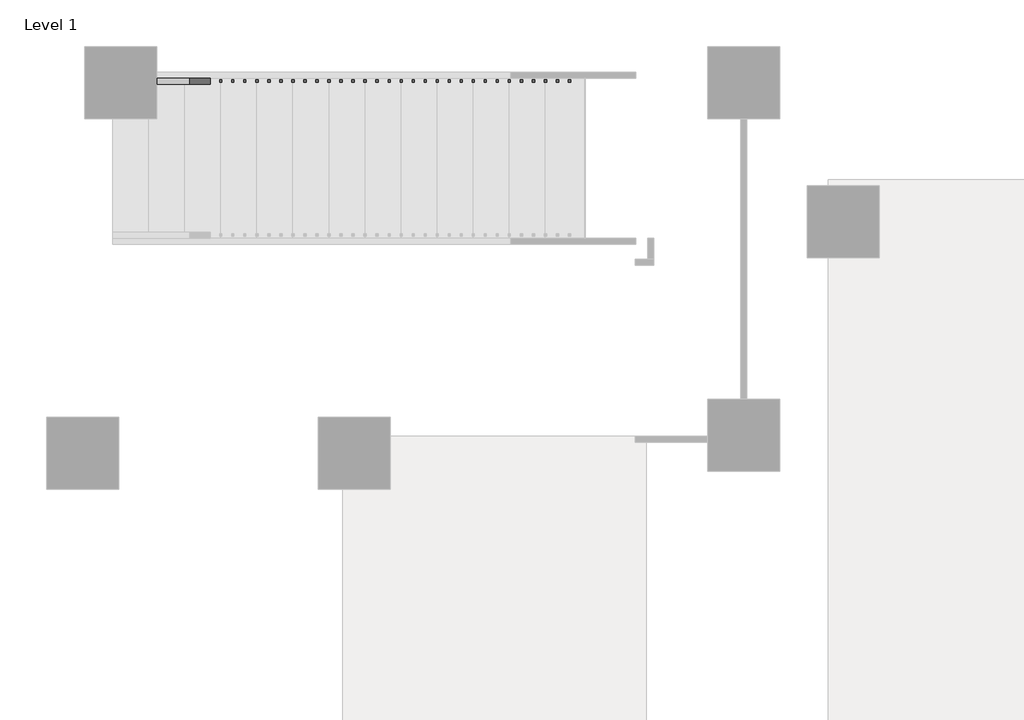
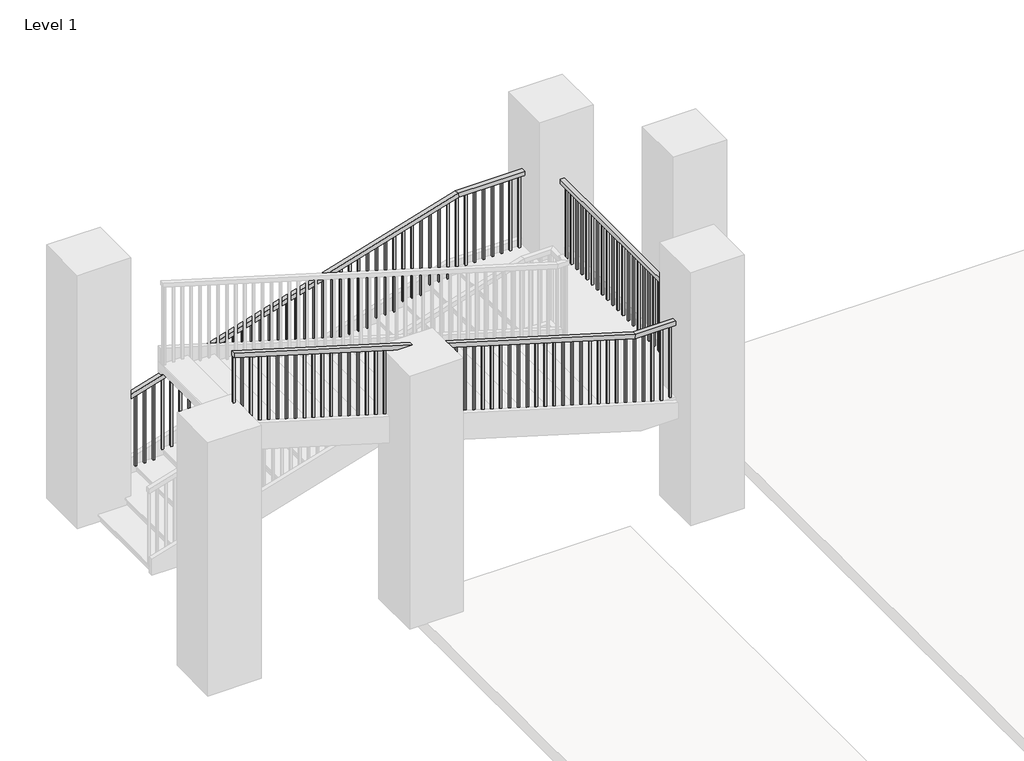
# One storey, part 5 of 6: 1 railing.
"""IFC4 building model written with IfcOpenShell, lengths in millimetres."""

from ifc_helpers import new_model, si_unit, frame, origin, place, context, project, spatial, polyline, outline, extrude, faceted_brep, element, save

model = new_model("IFC4")

# Units and contexts
model_context = context("Model", 3, world=origin())
ifc_project = project(units=[si_unit("LENGTHUNIT", "METRE", prefix="MILLI")], contexts=[model_context])

# Site, building, storey
site = spatial("IfcSite", under=ifc_project)
building = spatial("IfcBuilding", under=site)
storey = spatial("IfcBuildingStorey", under=building, Name="Level 1", Elevation=0.0)

# Railing
placement = place(None, origin())
element("IfcRailing", 1, ObjectType="Handrail - Rectangular", at=placement, inside=storey, context=model_context, shape_type="SolidModel", body=[
    faceted_brep([(-5254.0891351, 12506.0715905, 1005.84), (-5254.0891351, 12506.0715905, 952.8032429), (-5254.0891351, 12455.2715905, 952.8032429), (-5254.0891351, 12455.2715905, 1005.84), (-986.8891351, 12506.0715905, 2286.0), (-979.4332782, 12506.0715905, 2235.2), (-979.4332782, 12455.2715905, 2235.2), (-986.8891351, 12455.2715905, 2286.0), (54.5108649, 12506.0715905, 2286.0), (54.5108649, 12506.0715905, 2235.2), (3.7108649, 12455.2715905, 2235.2), (3.7108649, 12455.2715905, 2286.0), (54.5108649, 9478.4949943, 2286.0), (54.5108649, 9478.4949943, 2235.2), (3.7108649, 9529.2949943, 2235.2), (3.7108649, 9529.2949943, 2286.0), (-682.0891351, 9478.4949943, 2286.0), (-689.544992, 9478.4949943, 2235.2), (-689.544992, 9529.2949943, 2235.2), (-682.0891351, 9529.2949943, 2286.0), (-5254.0891351, 9478.4949943, 3657.6), (-5254.0891351, 9529.2949943, 3657.6), (-5254.0891351, 9529.2949943, 3604.5632429), (-5254.0891351, 9478.4949943, 3604.5632429)], [[[0, 1, 2, 3]], [[1, 0, 4, 5]], [[2, 1, 5, 6]], [[3, 2, 6, 7]], [[0, 3, 7, 4]], [[5, 4, 8, 9]], [[6, 5, 9, 10]], [[7, 6, 10, 11]], [[4, 7, 11, 8]], [[9, 8, 12, 13]], [[10, 9, 13, 14]], [[11, 10, 14, 15]], [[8, 11, 15, 12]], [[13, 12, 16, 17]], [[14, 13, 17, 18]], [[15, 14, 18, 19]], [[12, 15, 19, 16]], [[20, 21, 22, 23]], [[17, 16, 20, 23]], [[18, 17, 23, 22]], [[19, 18, 22, 21]], [[16, 19, 21, 20]]]),
    extrude(outline(polyline([(3576.9407429, -5162.0141351), (2651.76, -5162.0141351), (2651.76, -5142.9641351), (3571.2257429, -5142.9641351), (3576.9407429, -5162.0141351)])), frame((0.0, 9494.3699943, 0.0), z_axis=(0.0, 1.0, 0.0), x_axis=(0.0, 0.0, 1.0)), (0.0, 0.0, 1.0), 19.05),
    extrude(outline(polyline([(3546.4607429, -5060.4141351), (2651.76, -5060.4141351), (2651.76, -5041.3641351), (3540.7457429, -5041.3641351), (3546.4607429, -5060.4141351)])), frame((0.0, 9494.3699943, 0.0), z_axis=(0.0, 1.0, 0.0), x_axis=(0.0, 0.0, 1.0)), (0.0, 0.0, 1.0), 19.05),
    extrude(outline(polyline([(3515.9807429, -4958.8141351), (2651.76, -4958.8141351), (2651.76, -4939.7641351), (3510.2657429, -4939.7641351), (3515.9807429, -4958.8141351)])), frame((0.0, 9494.3699943, 0.0), z_axis=(0.0, 1.0, 0.0), x_axis=(0.0, 0.0, 1.0)), (0.0, 0.0, 1.0), 19.05),
    extrude(outline(polyline([(3485.5007429, -4857.2141351), (2560.32, -4857.2141351), (2560.32, -4838.1641351), (3479.7857429, -4838.1641351), (3485.5007429, -4857.2141351)])), frame((0.0, 9494.3699943, 0.0), z_axis=(0.0, 1.0, 0.0), x_axis=(0.0, 0.0, 1.0)), (0.0, 0.0, 1.0), 19.05),
    extrude(outline(polyline([(3455.0207429, -4755.6141351), (2560.32, -4755.6141351), (2560.32, -4736.5641351), (3449.3057429, -4736.5641351), (3455.0207429, -4755.6141351)])), frame((0.0, 9494.3699943, 0.0), z_axis=(0.0, 1.0, 0.0), x_axis=(0.0, 0.0, 1.0)), (0.0, 0.0, 1.0), 19.05),
    extrude(outline(polyline([(3424.5407429, -4654.0141351), (2560.32, -4654.0141351), (2560.32, -4634.9641351), (3418.8257429, -4634.9641351), (3424.5407429, -4654.0141351)])), frame((0.0, 9494.3699943, 0.0), z_axis=(0.0, 1.0, 0.0), x_axis=(0.0, 0.0, 1.0)), (0.0, 0.0, 1.0), 19.05),
    extrude(outline(polyline([(3394.0607429, -4552.4141351), (2468.88, -4552.4141351), (2468.88, -4533.3641351), (3388.3457429, -4533.3641351), (3394.0607429, -4552.4141351)])), frame((0.0, 9494.3699943, 0.0), z_axis=(0.0, 1.0, 0.0), x_axis=(0.0, 0.0, 1.0)), (0.0, 0.0, 1.0), 19.05),
    extrude(outline(polyline([(3363.5807429, -4450.8141351), (2468.88, -4450.8141351), (2468.88, -4431.7641351), (3357.8657429, -4431.7641351), (3363.5807429, -4450.8141351)])), frame((0.0, 9494.3699943, 0.0), z_axis=(0.0, 1.0, 0.0), x_axis=(0.0, 0.0, 1.0)), (0.0, 0.0, 1.0), 19.05),
    extrude(outline(polyline([(3333.1007429, -4349.2141351), (2468.88, -4349.2141351), (2468.88, -4330.1641351), (3327.3857429, -4330.1641351), (3333.1007429, -4349.2141351)])), frame((0.0, 9494.3699943, 0.0), z_axis=(0.0, 1.0, 0.0), x_axis=(0.0, 0.0, 1.0)), (0.0, 0.0, 1.0), 19.05),
    extrude(outline(polyline([(3302.6207429, -4247.6141351), (2377.44, -4247.6141351), (2377.44, -4228.5641351), (3296.9057429, -4228.5641351), (3302.6207429, -4247.6141351)])), frame((0.0, 9494.3699943, 0.0), z_axis=(0.0, 1.0, 0.0), x_axis=(0.0, 0.0, 1.0)), (0.0, 0.0, 1.0), 19.05),
    extrude(outline(polyline([(3272.1407429, -4146.0141351), (2377.44, -4146.0141351), (2377.44, -4126.9641351), (3266.4257429, -4126.9641351), (3272.1407429, -4146.0141351)])), frame((0.0, 9494.3699943, 0.0), z_axis=(0.0, 1.0, 0.0), x_axis=(0.0, 0.0, 1.0)), (0.0, 0.0, 1.0), 19.05),
    extrude(outline(polyline([(3241.6607429, -4044.4141351), (2377.44, -4044.4141351), (2377.44, -4025.3641351), (3235.9457429, -4025.3641351), (3241.6607429, -4044.4141351)])), frame((0.0, 9494.3699943, 0.0), z_axis=(0.0, 1.0, 0.0), x_axis=(0.0, 0.0, 1.0)), (0.0, 0.0, 1.0), 19.05),
    extrude(outline(polyline([(3211.1807429, -3942.8141351), (2286.0, -3942.8141351), (2286.0, -3923.7641351), (3205.4657429, -3923.7641351), (3211.1807429, -3942.8141351)])), frame((0.0, 9494.3699943, 0.0), z_axis=(0.0, 1.0, 0.0), x_axis=(0.0, 0.0, 1.0)), (0.0, 0.0, 1.0), 19.05),
    extrude(outline(polyline([(3180.7007429, -3841.2141351), (2286.0, -3841.2141351), (2286.0, -3822.1641351), (3174.9857429, -3822.1641351), (3180.7007429, -3841.2141351)])), frame((0.0, 9494.3699943, 0.0), z_axis=(0.0, 1.0, 0.0), x_axis=(0.0, 0.0, 1.0)), (0.0, 0.0, 1.0), 19.05),
    extrude(outline(polyline([(3150.2207429, -3739.6141351), (2286.0, -3739.6141351), (2286.0, -3720.5641351), (3144.5057429, -3720.5641351), (3150.2207429, -3739.6141351)])), frame((0.0, 9494.3699943, 0.0), z_axis=(0.0, 1.0, 0.0), x_axis=(0.0, 0.0, 1.0)), (0.0, 0.0, 1.0), 19.05),
    extrude(outline(polyline([(3119.7407429, -3638.0141351), (2194.56, -3638.0141351), (2194.56, -3618.9641351), (3114.0257429, -3618.9641351), (3119.7407429, -3638.0141351)])), frame((0.0, 9494.3699943, 0.0), z_axis=(0.0, 1.0, 0.0), x_axis=(0.0, 0.0, 1.0)), (0.0, 0.0, 1.0), 19.05),
    extrude(outline(polyline([(3089.2607429, -3536.4141351), (2194.56, -3536.4141351), (2194.56, -3517.3641351), (3083.5457429, -3517.3641351), (3089.2607429, -3536.4141351)])), frame((0.0, 9494.3699943, 0.0), z_axis=(0.0, 1.0, 0.0), x_axis=(0.0, 0.0, 1.0)), (0.0, 0.0, 1.0), 19.05),
    extrude(outline(polyline([(3058.7807429, -3434.8141351), (2194.56, -3434.8141351), (2194.56, -3415.7641351), (3053.0657429, -3415.7641351), (3058.7807429, -3434.8141351)])), frame((0.0, 9494.3699943, 0.0), z_axis=(0.0, 1.0, 0.0), x_axis=(0.0, 0.0, 1.0)), (0.0, 0.0, 1.0), 19.05),
    extrude(outline(polyline([(3028.3007429, -3333.2141351), (2103.12, -3333.2141351), (2103.12, -3314.1641351), (3022.5857429, -3314.1641351), (3028.3007429, -3333.2141351)])), frame((0.0, 9494.3699943, 0.0), z_axis=(0.0, 1.0, 0.0), x_axis=(0.0, 0.0, 1.0)), (0.0, 0.0, 1.0), 19.05),
    extrude(outline(polyline([(2997.8207429, -3231.6141351), (2103.12, -3231.6141351), (2103.12, -3212.5641351), (2992.1057429, -3212.5641351), (2997.8207429, -3231.6141351)])), frame((0.0, 9494.3699943, 0.0), z_axis=(0.0, 1.0, 0.0), x_axis=(0.0, 0.0, 1.0)), (0.0, 0.0, 1.0), 19.05),
    extrude(outline(polyline([(2967.3407429, -3130.0141351), (2103.12, -3130.0141351), (2103.12, -3110.9641351), (2961.6257429, -3110.9641351), (2967.3407429, -3130.0141351)])), frame((0.0, 9494.3699943, 0.0), z_axis=(0.0, 1.0, 0.0), x_axis=(0.0, 0.0, 1.0)), (0.0, 0.0, 1.0), 19.05),
    extrude(outline(polyline([(2936.8607429, -3028.4141351), (2011.68, -3028.4141351), (2011.68, -3009.3641351), (2931.1457429, -3009.3641351), (2936.8607429, -3028.4141351)])), frame((0.0, 9494.3699943, 0.0), z_axis=(0.0, 1.0, 0.0), x_axis=(0.0, 0.0, 1.0)), (0.0, 0.0, 1.0), 19.05),
    extrude(outline(polyline([(2906.3807429, -2926.8141351), (2011.68, -2926.8141351), (2011.68, -2907.7641351), (2900.6657429, -2907.7641351), (2906.3807429, -2926.8141351)])), frame((0.0, 9494.3699943, 0.0), z_axis=(0.0, 1.0, 0.0), x_axis=(0.0, 0.0, 1.0)), (0.0, 0.0, 1.0), 19.05),
    extrude(outline(polyline([(2875.9007429, -2825.2141351), (2011.68, -2825.2141351), (2011.68, -2806.1641351), (2870.1857429, -2806.1641351), (2875.9007429, -2825.2141351)])), frame((0.0, 9494.3699943, 0.0), z_axis=(0.0, 1.0, 0.0), x_axis=(0.0, 0.0, 1.0)), (0.0, 0.0, 1.0), 19.05),
    extrude(outline(polyline([(2845.4207429, -2723.6141351), (1920.24, -2723.6141351), (1920.24, -2704.5641351), (2839.7057429, -2704.5641351), (2845.4207429, -2723.6141351)])), frame((0.0, 9494.3699943, 0.0), z_axis=(0.0, 1.0, 0.0), x_axis=(0.0, 0.0, 1.0)), (0.0, 0.0, 1.0), 19.05),
    extrude(outline(polyline([(2814.9407429, -2622.0141351), (1920.24, -2622.0141351), (1920.24, -2602.9641351), (2809.2257429, -2602.9641351), (2814.9407429, -2622.0141351)])), frame((0.0, 9494.3699943, 0.0), z_axis=(0.0, 1.0, 0.0), x_axis=(0.0, 0.0, 1.0)), (0.0, 0.0, 1.0), 19.05),
    extrude(outline(polyline([(2784.4607429, -2520.4141351), (1920.24, -2520.4141351), (1920.24, -2501.3641351), (2778.7457429, -2501.3641351), (2784.4607429, -2520.4141351)])), frame((0.0, 9494.3699943, 0.0), z_axis=(0.0, 1.0, 0.0), x_axis=(0.0, 0.0, 1.0)), (0.0, 0.0, 1.0), 19.05),
    extrude(outline(polyline([(2753.9807429, -2418.8141351), (1828.8, -2418.8141351), (1828.8, -2399.7641351), (2748.2657429, -2399.7641351), (2753.9807429, -2418.8141351)])), frame((0.0, 9494.3699943, 0.0), z_axis=(0.0, 1.0, 0.0), x_axis=(0.0, 0.0, 1.0)), (0.0, 0.0, 1.0), 19.05),
    extrude(outline(polyline([(2723.5007429, -2317.2141351), (1828.8, -2317.2141351), (1828.8, -2298.1641351), (2717.7857429, -2298.1641351), (2723.5007429, -2317.2141351)])), frame((0.0, 9494.3699943, 0.0), z_axis=(0.0, 1.0, 0.0), x_axis=(0.0, 0.0, 1.0)), (0.0, 0.0, 1.0), 19.05),
    extrude(outline(polyline([(2693.0207429, -2215.6141351), (1828.8, -2215.6141351), (1828.8, -2196.5641351), (2687.3057429, -2196.5641351), (2693.0207429, -2215.6141351)])), frame((0.0, 9494.3699943, 0.0), z_axis=(0.0, 1.0, 0.0), x_axis=(0.0, 0.0, 1.0)), (0.0, 0.0, 1.0), 19.05),
    extrude(outline(polyline([(2662.5407429, -2114.0141351), (1737.36, -2114.0141351), (1737.36, -2094.9641351), (2656.8257429, -2094.9641351), (2662.5407429, -2114.0141351)])), frame((0.0, 9494.3699943, 0.0), z_axis=(0.0, 1.0, 0.0), x_axis=(0.0, 0.0, 1.0)), (0.0, 0.0, 1.0), 19.05),
    extrude(outline(polyline([(2632.0607429, -2012.4141351), (1737.36, -2012.4141351), (1737.36, -1993.3641351), (2626.3457429, -1993.3641351), (2632.0607429, -2012.4141351)])), frame((0.0, 9494.3699943, 0.0), z_axis=(0.0, 1.0, 0.0), x_axis=(0.0, 0.0, 1.0)), (0.0, 0.0, 1.0), 19.05),
    extrude(outline(polyline([(2601.5807429, -1910.8141351), (1737.36, -1910.8141351), (1737.36, -1891.7641351), (2595.8657429, -1891.7641351), (2601.5807429, -1910.8141351)])), frame((0.0, 9494.3699943, 0.0), z_axis=(0.0, 1.0, 0.0), x_axis=(0.0, 0.0, 1.0)), (0.0, 0.0, 1.0), 19.05),
    extrude(outline(polyline([(2571.1007429, -1809.2141351), (1645.92, -1809.2141351), (1645.92, -1790.1641351), (2565.3857429, -1790.1641351), (2571.1007429, -1809.2141351)])), frame((0.0, 9494.3699943, 0.0), z_axis=(0.0, 1.0, 0.0), x_axis=(0.0, 0.0, 1.0)), (0.0, 0.0, 1.0), 19.05),
    extrude(outline(polyline([(2540.6207429, -1707.6141351), (1645.92, -1707.6141351), (1645.92, -1688.5641351), (2534.9057429, -1688.5641351), (2540.6207429, -1707.6141351)])), frame((0.0, 9494.3699943, 0.0), z_axis=(0.0, 1.0, 0.0), x_axis=(0.0, 0.0, 1.0)), (0.0, 0.0, 1.0), 19.05),
    extrude(outline(polyline([(2510.1407429, -1606.0141351), (1645.92, -1606.0141351), (1645.92, -1586.9641351), (2504.4257429, -1586.9641351), (2510.1407429, -1606.0141351)])), frame((0.0, 9494.3699943, 0.0), z_axis=(0.0, 1.0, 0.0), x_axis=(0.0, 0.0, 1.0)), (0.0, 0.0, 1.0), 19.05),
    extrude(outline(polyline([(2479.6607429, -1504.4141351), (1554.48, -1504.4141351), (1554.48, -1485.3641351), (2473.9457429, -1485.3641351), (2479.6607429, -1504.4141351)])), frame((0.0, 9494.3699943, 0.0), z_axis=(0.0, 1.0, 0.0), x_axis=(0.0, 0.0, 1.0)), (0.0, 0.0, 1.0), 19.05),
    extrude(outline(polyline([(2449.1807429, -1402.8141351), (1554.48, -1402.8141351), (1554.48, -1383.7641351), (2443.4657429, -1383.7641351), (2449.1807429, -1402.8141351)])), frame((0.0, 9494.3699943, 0.0), z_axis=(0.0, 1.0, 0.0), x_axis=(0.0, 0.0, 1.0)), (0.0, 0.0, 1.0), 19.05),
    extrude(outline(polyline([(2418.7007429, -1301.2141351), (1554.48, -1301.2141351), (1554.48, -1282.1641351), (2412.9857429, -1282.1641351), (2418.7007429, -1301.2141351)])), frame((0.0, 9494.3699943, 0.0), z_axis=(0.0, 1.0, 0.0), x_axis=(0.0, 0.0, 1.0)), (0.0, 0.0, 1.0), 19.05),
    extrude(outline(polyline([(2388.2207429, -1199.6141351), (1463.04, -1199.6141351), (1463.04, -1180.5641351), (2382.5057429, -1180.5641351), (2388.2207429, -1199.6141351)])), frame((0.0, 9494.3699943, 0.0), z_axis=(0.0, 1.0, 0.0), x_axis=(0.0, 0.0, 1.0)), (0.0, 0.0, 1.0), 19.05),
    extrude(outline(polyline([(2357.7407429, -1098.0141351), (1463.04, -1098.0141351), (1463.04, -1078.9641351), (2352.0257429, -1078.9641351), (2357.7407429, -1098.0141351)])), frame((0.0, 9494.3699943, 0.0), z_axis=(0.0, 1.0, 0.0), x_axis=(0.0, 0.0, 1.0)), (0.0, 0.0, 1.0), 19.05),
    extrude(outline(polyline([(2327.2607429, -996.4141351), (1463.04, -996.4141351), (1463.04, -977.3641351), (2321.5457429, -977.3641351), (2327.2607429, -996.4141351)])), frame((0.0, 9494.3699943, 0.0), z_axis=(0.0, 1.0, 0.0), x_axis=(0.0, 0.0, 1.0)), (0.0, 0.0, 1.0), 19.05),
    extrude(outline(polyline([(2296.7807429, -894.8141351), (1371.6, -894.8141351), (1371.6, -875.7641351), (2291.0657429, -875.7641351), (2296.7807429, -894.8141351)])), frame((0.0, 9494.3699943, 0.0), z_axis=(0.0, 1.0, 0.0), x_axis=(0.0, 0.0, 1.0)), (0.0, 0.0, 1.0), 19.05),
    extrude(outline(polyline([(2266.3007429, -793.2141351), (1371.6, -793.2141351), (1371.6, -774.1641351), (2260.5857429, -774.1641351), (2266.3007429, -793.2141351)])), frame((0.0, 9494.3699943, 0.0), z_axis=(0.0, 1.0, 0.0), x_axis=(0.0, 0.0, 1.0)), (0.0, 0.0, 1.0), 19.05),
    extrude(outline(polyline([(-672.5641351, 9494.3699943), (-691.6141351, 9494.3699943), (-691.6141351, 9513.4199943), (-672.5641351, 9513.4199943), (-672.5641351, 9494.3699943)])), frame((0.0, 0.0, 1371.6), z_axis=(0.0, 0.0, 1.0), x_axis=(1.0, 0.0, 0.0)), (0.0, 0.0, 1.0), 863.6),
    extrude(outline(polyline([(-570.9641351, 9494.3699943), (-590.0141351, 9494.3699943), (-590.0141351, 9513.4199943), (-570.9641351, 9513.4199943), (-570.9641351, 9494.3699943)])), frame((0.0, 0.0, 1371.6), z_axis=(0.0, 0.0, 1.0), x_axis=(1.0, 0.0, 0.0)), (0.0, 0.0, 1.0), 863.6),
    extrude(outline(polyline([(-469.3641351, 9494.3699943), (-488.4141351, 9494.3699943), (-488.4141351, 9513.4199943), (-469.3641351, 9513.4199943), (-469.3641351, 9494.3699943)])), frame((0.0, 0.0, 1371.6), z_axis=(0.0, 0.0, 1.0), x_axis=(1.0, 0.0, 0.0)), (0.0, 0.0, 1.0), 863.6),
    extrude(outline(polyline([(-367.7641351, 9494.3699943), (-386.8141351, 9494.3699943), (-386.8141351, 9513.4199943), (-367.7641351, 9513.4199943), (-367.7641351, 9494.3699943)])), frame((0.0, 0.0, 1371.6), z_axis=(0.0, 0.0, 1.0), x_axis=(1.0, 0.0, 0.0)), (0.0, 0.0, 1.0), 863.6),
    extrude(outline(polyline([(-266.1641351, 9494.3699943), (-285.2141351, 9494.3699943), (-285.2141351, 9513.4199943), (-266.1641351, 9513.4199943), (-266.1641351, 9494.3699943)])), frame((0.0, 0.0, 1371.6), z_axis=(0.0, 0.0, 1.0), x_axis=(1.0, 0.0, 0.0)), (0.0, 0.0, 1.0), 863.6),
    extrude(outline(polyline([(-164.5641351, 9494.3699943), (-183.6141351, 9494.3699943), (-183.6141351, 9513.4199943), (-164.5641351, 9513.4199943), (-164.5641351, 9494.3699943)])), frame((0.0, 0.0, 1371.6), z_axis=(0.0, 0.0, 1.0), x_axis=(1.0, 0.0, 0.0)), (0.0, 0.0, 1.0), 863.6),
    extrude(outline(polyline([(-62.9641351, 9494.3699943), (-82.0141351, 9494.3699943), (-82.0141351, 9513.4199943), (-62.9641351, 9513.4199943), (-62.9641351, 9494.3699943)])), frame((0.0, 0.0, 1371.6), z_axis=(0.0, 0.0, 1.0), x_axis=(1.0, 0.0, 0.0)), (0.0, 0.0, 1.0), 863.6),
    extrude(outline(polyline([(38.6358649, 9543.7965905), (38.6358649, 9524.7465905), (19.5858649, 9524.7465905), (19.5858649, 9543.7965905), (38.6358649, 9543.7965905)])), frame((0.0, 0.0, 1371.6), z_axis=(0.0, 0.0, 1.0), x_axis=(1.0, 0.0, 0.0)), (0.0, 0.0, 1.0), 863.6),
    extrude(outline(polyline([(38.6358649, 9645.3965905), (38.6358649, 9626.3465905), (19.5858649, 9626.3465905), (19.5858649, 9645.3965905), (38.6358649, 9645.3965905)])), frame((0.0, 0.0, 1371.6), z_axis=(0.0, 0.0, 1.0), x_axis=(1.0, 0.0, 0.0)), (0.0, 0.0, 1.0), 863.6),
    extrude(outline(polyline([(38.6358649, 9746.9965905), (38.6358649, 9727.9465905), (19.5858649, 9727.9465905), (19.5858649, 9746.9965905), (38.6358649, 9746.9965905)])), frame((0.0, 0.0, 1371.6), z_axis=(0.0, 0.0, 1.0), x_axis=(1.0, 0.0, 0.0)), (0.0, 0.0, 1.0), 863.6),
    extrude(outline(polyline([(38.6358649, 9848.5965905), (38.6358649, 9829.5465905), (19.5858649, 9829.5465905), (19.5858649, 9848.5965905), (38.6358649, 9848.5965905)])), frame((0.0, 0.0, 1371.6), z_axis=(0.0, 0.0, 1.0), x_axis=(1.0, 0.0, 0.0)), (0.0, 0.0, 1.0), 863.6),
    extrude(outline(polyline([(38.6358649, 9950.1965905), (38.6358649, 9931.1465905), (19.5858649, 9931.1465905), (19.5858649, 9950.1965905), (38.6358649, 9950.1965905)])), frame((0.0, 0.0, 1371.6), z_axis=(0.0, 0.0, 1.0), x_axis=(1.0, 0.0, 0.0)), (0.0, 0.0, 1.0), 863.6),
    extrude(outline(polyline([(38.6358649, 10051.7965905), (38.6358649, 10032.7465905), (19.5858649, 10032.7465905), (19.5858649, 10051.7965905), (38.6358649, 10051.7965905)])), frame((0.0, 0.0, 1371.6), z_axis=(0.0, 0.0, 1.0), x_axis=(1.0, 0.0, 0.0)), (0.0, 0.0, 1.0), 863.6),
    extrude(outline(polyline([(38.6358649, 10153.3965905), (38.6358649, 10134.3465905), (19.5858649, 10134.3465905), (19.5858649, 10153.3965905), (38.6358649, 10153.3965905)])), frame((0.0, 0.0, 1371.6), z_axis=(0.0, 0.0, 1.0), x_axis=(1.0, 0.0, 0.0)), (0.0, 0.0, 1.0), 863.6),
    extrude(outline(polyline([(38.6358649, 10254.9965905), (38.6358649, 10235.9465905), (19.5858649, 10235.9465905), (19.5858649, 10254.9965905), (38.6358649, 10254.9965905)])), frame((0.0, 0.0, 1371.6), z_axis=(0.0, 0.0, 1.0), x_axis=(1.0, 0.0, 0.0)), (0.0, 0.0, 1.0), 863.6),
    extrude(outline(polyline([(38.6358649, 10356.5965905), (38.6358649, 10337.5465905), (19.5858649, 10337.5465905), (19.5858649, 10356.5965905), (38.6358649, 10356.5965905)])), frame((0.0, 0.0, 1371.6), z_axis=(0.0, 0.0, 1.0), x_axis=(1.0, 0.0, 0.0)), (0.0, 0.0, 1.0), 863.6),
    extrude(outline(polyline([(38.6358649, 10458.1965905), (38.6358649, 10439.1465905), (19.5858649, 10439.1465905), (19.5858649, 10458.1965905), (38.6358649, 10458.1965905)])), frame((0.0, 0.0, 1371.6), z_axis=(0.0, 0.0, 1.0), x_axis=(1.0, 0.0, 0.0)), (0.0, 0.0, 1.0), 863.6),
    extrude(outline(polyline([(38.6358649, 10559.7965905), (38.6358649, 10540.7465905), (19.5858649, 10540.7465905), (19.5858649, 10559.7965905), (38.6358649, 10559.7965905)])), frame((0.0, 0.0, 1371.6), z_axis=(0.0, 0.0, 1.0), x_axis=(1.0, 0.0, 0.0)), (0.0, 0.0, 1.0), 863.6),
    extrude(outline(polyline([(38.6358649, 10661.3965905), (38.6358649, 10642.3465905), (19.5858649, 10642.3465905), (19.5858649, 10661.3965905), (38.6358649, 10661.3965905)])), frame((0.0, 0.0, 1371.6), z_axis=(0.0, 0.0, 1.0), x_axis=(1.0, 0.0, 0.0)), (0.0, 0.0, 1.0), 863.6),
    extrude(outline(polyline([(38.6358649, 10762.9965905), (38.6358649, 10743.9465905), (19.5858649, 10743.9465905), (19.5858649, 10762.9965905), (38.6358649, 10762.9965905)])), frame((0.0, 0.0, 1371.6), z_axis=(0.0, 0.0, 1.0), x_axis=(1.0, 0.0, 0.0)), (0.0, 0.0, 1.0), 863.6),
    extrude(outline(polyline([(38.6358649, 10864.5965905), (38.6358649, 10845.5465905), (19.5858649, 10845.5465905), (19.5858649, 10864.5965905), (38.6358649, 10864.5965905)])), frame((0.0, 0.0, 1371.6), z_axis=(0.0, 0.0, 1.0), x_axis=(1.0, 0.0, 0.0)), (0.0, 0.0, 1.0), 863.6),
    extrude(outline(polyline([(38.6358649, 10966.1965905), (38.6358649, 10947.1465905), (19.5858649, 10947.1465905), (19.5858649, 10966.1965905), (38.6358649, 10966.1965905)])), frame((0.0, 0.0, 1371.6), z_axis=(0.0, 0.0, 1.0), x_axis=(1.0, 0.0, 0.0)), (0.0, 0.0, 1.0), 863.6),
    extrude(outline(polyline([(38.6358649, 11067.7965905), (38.6358649, 11048.7465905), (19.5858649, 11048.7465905), (19.5858649, 11067.7965905), (38.6358649, 11067.7965905)])), frame((0.0, 0.0, 1371.6), z_axis=(0.0, 0.0, 1.0), x_axis=(1.0, 0.0, 0.0)), (0.0, 0.0, 1.0), 863.6),
    extrude(outline(polyline([(38.6358649, 11169.3965905), (38.6358649, 11150.3465905), (19.5858649, 11150.3465905), (19.5858649, 11169.3965905), (38.6358649, 11169.3965905)])), frame((0.0, 0.0, 1371.6), z_axis=(0.0, 0.0, 1.0), x_axis=(1.0, 0.0, 0.0)), (0.0, 0.0, 1.0), 863.6),
    extrude(outline(polyline([(38.6358649, 11270.9965905), (38.6358649, 11251.9465905), (19.5858649, 11251.9465905), (19.5858649, 11270.9965905), (38.6358649, 11270.9965905)])), frame((0.0, 0.0, 1371.6), z_axis=(0.0, 0.0, 1.0), x_axis=(1.0, 0.0, 0.0)), (0.0, 0.0, 1.0), 863.6),
    extrude(outline(polyline([(38.6358649, 11372.5965905), (38.6358649, 11353.5465905), (19.5858649, 11353.5465905), (19.5858649, 11372.5965905), (38.6358649, 11372.5965905)])), frame((0.0, 0.0, 1371.6), z_axis=(0.0, 0.0, 1.0), x_axis=(1.0, 0.0, 0.0)), (0.0, 0.0, 1.0), 863.6),
    extrude(outline(polyline([(38.6358649, 11474.1965905), (38.6358649, 11455.1465905), (19.5858649, 11455.1465905), (19.5858649, 11474.1965905), (38.6358649, 11474.1965905)])), frame((0.0, 0.0, 1371.6), z_axis=(0.0, 0.0, 1.0), x_axis=(1.0, 0.0, 0.0)), (0.0, 0.0, 1.0), 863.6),
    extrude(outline(polyline([(38.6358649, 11575.7965905), (38.6358649, 11556.7465905), (19.5858649, 11556.7465905), (19.5858649, 11575.7965905), (38.6358649, 11575.7965905)])), frame((0.0, 0.0, 1371.6), z_axis=(0.0, 0.0, 1.0), x_axis=(1.0, 0.0, 0.0)), (0.0, 0.0, 1.0), 863.6),
    extrude(outline(polyline([(38.6358649, 11677.3965905), (38.6358649, 11658.3465905), (19.5858649, 11658.3465905), (19.5858649, 11677.3965905), (38.6358649, 11677.3965905)])), frame((0.0, 0.0, 1371.6), z_axis=(0.0, 0.0, 1.0), x_axis=(1.0, 0.0, 0.0)), (0.0, 0.0, 1.0), 863.6),
    extrude(outline(polyline([(38.6358649, 11778.9965905), (38.6358649, 11759.9465905), (19.5858649, 11759.9465905), (19.5858649, 11778.9965905), (38.6358649, 11778.9965905)])), frame((0.0, 0.0, 1371.6), z_axis=(0.0, 0.0, 1.0), x_axis=(1.0, 0.0, 0.0)), (0.0, 0.0, 1.0), 863.6),
    extrude(outline(polyline([(38.6358649, 11880.5965905), (38.6358649, 11861.5465905), (19.5858649, 11861.5465905), (19.5858649, 11880.5965905), (38.6358649, 11880.5965905)])), frame((0.0, 0.0, 1371.6), z_axis=(0.0, 0.0, 1.0), x_axis=(1.0, 0.0, 0.0)), (0.0, 0.0, 1.0), 863.6),
    extrude(outline(polyline([(38.6358649, 11982.1965905), (38.6358649, 11963.1465905), (19.5858649, 11963.1465905), (19.5858649, 11982.1965905), (38.6358649, 11982.1965905)])), frame((0.0, 0.0, 1371.6), z_axis=(0.0, 0.0, 1.0), x_axis=(1.0, 0.0, 0.0)), (0.0, 0.0, 1.0), 863.6),
    extrude(outline(polyline([(38.6358649, 12083.7965905), (38.6358649, 12064.7465905), (19.5858649, 12064.7465905), (19.5858649, 12083.7965905), (38.6358649, 12083.7965905)])), frame((0.0, 0.0, 1371.6), z_axis=(0.0, 0.0, 1.0), x_axis=(1.0, 0.0, 0.0)), (0.0, 0.0, 1.0), 863.6),
    extrude(outline(polyline([(38.6358649, 12185.3965905), (38.6358649, 12166.3465905), (19.5858649, 12166.3465905), (19.5858649, 12185.3965905), (38.6358649, 12185.3965905)])), frame((0.0, 0.0, 1371.6), z_axis=(0.0, 0.0, 1.0), x_axis=(1.0, 0.0, 0.0)), (0.0, 0.0, 1.0), 863.6),
    extrude(outline(polyline([(38.6358649, 12286.9965905), (38.6358649, 12267.9465905), (19.5858649, 12267.9465905), (19.5858649, 12286.9965905), (38.6358649, 12286.9965905)])), frame((0.0, 0.0, 1371.6), z_axis=(0.0, 0.0, 1.0), x_axis=(1.0, 0.0, 0.0)), (0.0, 0.0, 1.0), 863.6),
    extrude(outline(polyline([(38.6358649, 12388.5965905), (38.6358649, 12369.5465905), (19.5858649, 12369.5465905), (19.5858649, 12388.5965905), (38.6358649, 12388.5965905)])), frame((0.0, 0.0, 1371.6), z_axis=(0.0, 0.0, 1.0), x_axis=(1.0, 0.0, 0.0)), (0.0, 0.0, 1.0), 863.6),
    extrude(outline(polyline([(-82.0141351, 12490.1965905), (-62.9641351, 12490.1965905), (-62.9641351, 12471.1465905), (-82.0141351, 12471.1465905), (-82.0141351, 12490.1965905)])), frame((0.0, 0.0, 1371.6), z_axis=(0.0, 0.0, 1.0), x_axis=(1.0, 0.0, 0.0)), (0.0, 0.0, 1.0), 863.6),
    extrude(outline(polyline([(-183.6141351, 12490.1965905), (-164.5641351, 12490.1965905), (-164.5641351, 12471.1465905), (-183.6141351, 12471.1465905), (-183.6141351, 12490.1965905)])), frame((0.0, 0.0, 1371.6), z_axis=(0.0, 0.0, 1.0), x_axis=(1.0, 0.0, 0.0)), (0.0, 0.0, 1.0), 863.6),
    extrude(outline(polyline([(-285.2141351, 12490.1965905), (-266.1641351, 12490.1965905), (-266.1641351, 12471.1465905), (-285.2141351, 12471.1465905), (-285.2141351, 12490.1965905)])), frame((0.0, 0.0, 1371.6), z_axis=(0.0, 0.0, 1.0), x_axis=(1.0, 0.0, 0.0)), (0.0, 0.0, 1.0), 863.6),
    extrude(outline(polyline([(-386.8141351, 12490.1965905), (-367.7641351, 12490.1965905), (-367.7641351, 12471.1465905), (-386.8141351, 12471.1465905), (-386.8141351, 12490.1965905)])), frame((0.0, 0.0, 1371.6), z_axis=(0.0, 0.0, 1.0), x_axis=(1.0, 0.0, 0.0)), (0.0, 0.0, 1.0), 863.6),
    extrude(outline(polyline([(-488.4141351, 12490.1965905), (-469.3641351, 12490.1965905), (-469.3641351, 12471.1465905), (-488.4141351, 12471.1465905), (-488.4141351, 12490.1965905)])), frame((0.0, 0.0, 1371.6), z_axis=(0.0, 0.0, 1.0), x_axis=(1.0, 0.0, 0.0)), (0.0, 0.0, 1.0), 863.6),
    extrude(outline(polyline([(-590.0141351, 12490.1965905), (-570.9641351, 12490.1965905), (-570.9641351, 12471.1465905), (-590.0141351, 12471.1465905), (-590.0141351, 12490.1965905)])), frame((0.0, 0.0, 1371.6), z_axis=(0.0, 0.0, 1.0), x_axis=(1.0, 0.0, 0.0)), (0.0, 0.0, 1.0), 863.6),
    extrude(outline(polyline([(-691.6141351, 12490.1965905), (-672.5641351, 12490.1965905), (-672.5641351, 12471.1465905), (-691.6141351, 12471.1465905), (-691.6141351, 12490.1965905)])), frame((0.0, 0.0, 1371.6), z_axis=(0.0, 0.0, 1.0), x_axis=(1.0, 0.0, 0.0)), (0.0, 0.0, 1.0), 863.6),
    extrude(outline(polyline([(-793.2141351, 12490.1965905), (-774.1641351, 12490.1965905), (-774.1641351, 12471.1465905), (-793.2141351, 12471.1465905), (-793.2141351, 12490.1965905)])), frame((0.0, 0.0, 1371.6), z_axis=(0.0, 0.0, 1.0), x_axis=(1.0, 0.0, 0.0)), (0.0, 0.0, 1.0), 863.6),
    extrude(outline(polyline([(-894.8141351, 12490.1965905), (-875.7641351, 12490.1965905), (-875.7641351, 12471.1465905), (-894.8141351, 12471.1465905), (-894.8141351, 12490.1965905)])), frame((0.0, 0.0, 1371.6), z_axis=(0.0, 0.0, 1.0), x_axis=(1.0, 0.0, 0.0)), (0.0, 0.0, 1.0), 863.6),
    extrude(outline(polyline([(2230.1057429, -996.4141351), (1371.6, -996.4141351), (1371.6, -977.3641351), (2235.8207429, -977.3641351), (2230.1057429, -996.4141351)])), frame((0.0, 12471.1465905, 0.0), z_axis=(0.0, 1.0, 0.0), x_axis=(0.0, 0.0, 1.0)), (0.0, 0.0, 1.0), 19.05),
    extrude(outline(polyline([(2199.6257429, -1098.0141351), (1280.16, -1098.0141351), (1280.16, -1078.9641351), (2205.3407429, -1078.9641351), (2199.6257429, -1098.0141351)])), frame((0.0, 12471.1465905, 0.0), z_axis=(0.0, 1.0, 0.0), x_axis=(0.0, 0.0, 1.0)), (0.0, 0.0, 1.0), 19.05),
    extrude(outline(polyline([(2169.1457429, -1199.6141351), (1280.16, -1199.6141351), (1280.16, -1180.5641351), (2174.8607429, -1180.5641351), (2169.1457429, -1199.6141351)])), frame((0.0, 12471.1465905, 0.0), z_axis=(0.0, 1.0, 0.0), x_axis=(0.0, 0.0, 1.0)), (0.0, 0.0, 1.0), 19.05),
    extrude(outline(polyline([(2138.6657429, -1301.2141351), (1280.16, -1301.2141351), (1280.16, -1282.1641351), (2144.3807429, -1282.1641351), (2138.6657429, -1301.2141351)])), frame((0.0, 12471.1465905, 0.0), z_axis=(0.0, 1.0, 0.0), x_axis=(0.0, 0.0, 1.0)), (0.0, 0.0, 1.0), 19.05),
    extrude(outline(polyline([(2108.1857429, -1402.8141351), (1188.72, -1402.8141351), (1188.72, -1383.7641351), (2113.9007429, -1383.7641351), (2108.1857429, -1402.8141351)])), frame((0.0, 12471.1465905, 0.0), z_axis=(0.0, 1.0, 0.0), x_axis=(0.0, 0.0, 1.0)), (0.0, 0.0, 1.0), 19.05),
    extrude(outline(polyline([(2077.7057429, -1504.4141351), (1188.72, -1504.4141351), (1188.72, -1485.3641351), (2083.4207429, -1485.3641351), (2077.7057429, -1504.4141351)])), frame((0.0, 12471.1465905, 0.0), z_axis=(0.0, 1.0, 0.0), x_axis=(0.0, 0.0, 1.0)), (0.0, 0.0, 1.0), 19.05),
    extrude(outline(polyline([(2047.2257429, -1606.0141351), (1188.72, -1606.0141351), (1188.72, -1586.9641351), (2052.9407429, -1586.9641351), (2047.2257429, -1606.0141351)])), frame((0.0, 12471.1465905, 0.0), z_axis=(0.0, 1.0, 0.0), x_axis=(0.0, 0.0, 1.0)), (0.0, 0.0, 1.0), 19.05),
    extrude(outline(polyline([(2016.7457429, -1707.6141351), (1097.28, -1707.6141351), (1097.28, -1688.5641351), (2022.4607429, -1688.5641351), (2016.7457429, -1707.6141351)])), frame((0.0, 12471.1465905, 0.0), z_axis=(0.0, 1.0, 0.0), x_axis=(0.0, 0.0, 1.0)), (0.0, 0.0, 1.0), 19.05),
    extrude(outline(polyline([(1986.2657429, -1809.2141351), (1097.28, -1809.2141351), (1097.28, -1790.1641351), (1991.9807429, -1790.1641351), (1986.2657429, -1809.2141351)])), frame((0.0, 12471.1465905, 0.0), z_axis=(0.0, 1.0, 0.0), x_axis=(0.0, 0.0, 1.0)), (0.0, 0.0, 1.0), 19.05),
    extrude(outline(polyline([(1955.7857429, -1910.8141351), (1097.28, -1910.8141351), (1097.28, -1891.7641351), (1961.5007429, -1891.7641351), (1955.7857429, -1910.8141351)])), frame((0.0, 12471.1465905, 0.0), z_axis=(0.0, 1.0, 0.0), x_axis=(0.0, 0.0, 1.0)), (0.0, 0.0, 1.0), 19.05),
    extrude(outline(polyline([(1925.3057429, -2012.4141351), (1005.84, -2012.4141351), (1005.84, -1993.3641351), (1931.0207429, -1993.3641351), (1925.3057429, -2012.4141351)])), frame((0.0, 12471.1465905, 0.0), z_axis=(0.0, 1.0, 0.0), x_axis=(0.0, 0.0, 1.0)), (0.0, 0.0, 1.0), 19.05),
    extrude(outline(polyline([(1894.8257429, -2114.0141351), (1005.84, -2114.0141351), (1005.84, -2094.9641351), (1900.5407429, -2094.9641351), (1894.8257429, -2114.0141351)])), frame((0.0, 12471.1465905, 0.0), z_axis=(0.0, 1.0, 0.0), x_axis=(0.0, 0.0, 1.0)), (0.0, 0.0, 1.0), 19.05),
    extrude(outline(polyline([(1864.3457429, -2215.6141351), (1005.84, -2215.6141351), (1005.84, -2196.5641351), (1870.0607429, -2196.5641351), (1864.3457429, -2215.6141351)])), frame((0.0, 12471.1465905, 0.0), z_axis=(0.0, 1.0, 0.0), x_axis=(0.0, 0.0, 1.0)), (0.0, 0.0, 1.0), 19.05),
    extrude(outline(polyline([(1833.8657429, -2317.2141351), (914.4, -2317.2141351), (914.4, -2298.1641351), (1839.5807429, -2298.1641351), (1833.8657429, -2317.2141351)])), frame((0.0, 12471.1465905, 0.0), z_axis=(0.0, 1.0, 0.0), x_axis=(0.0, 0.0, 1.0)), (0.0, 0.0, 1.0), 19.05),
    extrude(outline(polyline([(1803.3857429, -2418.8141351), (914.4, -2418.8141351), (914.4, -2399.7641351), (1809.1007429, -2399.7641351), (1803.3857429, -2418.8141351)])), frame((0.0, 12471.1465905, 0.0), z_axis=(0.0, 1.0, 0.0), x_axis=(0.0, 0.0, 1.0)), (0.0, 0.0, 1.0), 19.05),
    extrude(outline(polyline([(1772.9057429, -2520.4141351), (914.4, -2520.4141351), (914.4, -2501.3641351), (1778.6207429, -2501.3641351), (1772.9057429, -2520.4141351)])), frame((0.0, 12471.1465905, 0.0), z_axis=(0.0, 1.0, 0.0), x_axis=(0.0, 0.0, 1.0)), (0.0, 0.0, 1.0), 19.05),
    extrude(outline(polyline([(1742.4257429, -2622.0141351), (822.96, -2622.0141351), (822.96, -2602.9641351), (1748.1407429, -2602.9641351), (1742.4257429, -2622.0141351)])), frame((0.0, 12471.1465905, 0.0), z_axis=(0.0, 1.0, 0.0), x_axis=(0.0, 0.0, 1.0)), (0.0, 0.0, 1.0), 19.05),
    extrude(outline(polyline([(1711.9457429, -2723.6141351), (822.96, -2723.6141351), (822.96, -2704.5641351), (1717.6607429, -2704.5641351), (1711.9457429, -2723.6141351)])), frame((0.0, 12471.1465905, 0.0), z_axis=(0.0, 1.0, 0.0), x_axis=(0.0, 0.0, 1.0)), (0.0, 0.0, 1.0), 19.05),
    extrude(outline(polyline([(1681.4657429, -2825.2141351), (822.96, -2825.2141351), (822.96, -2806.1641351), (1687.1807429, -2806.1641351), (1681.4657429, -2825.2141351)])), frame((0.0, 12471.1465905, 0.0), z_axis=(0.0, 1.0, 0.0), x_axis=(0.0, 0.0, 1.0)), (0.0, 0.0, 1.0), 19.05),
    extrude(outline(polyline([(1650.9857429, -2926.8141351), (731.52, -2926.8141351), (731.52, -2907.7641351), (1656.7007429, -2907.7641351), (1650.9857429, -2926.8141351)])), frame((0.0, 12471.1465905, 0.0), z_axis=(0.0, 1.0, 0.0), x_axis=(0.0, 0.0, 1.0)), (0.0, 0.0, 1.0), 19.05),
    extrude(outline(polyline([(1620.5057429, -3028.4141351), (731.52, -3028.4141351), (731.52, -3009.3641351), (1626.2207429, -3009.3641351), (1620.5057429, -3028.4141351)])), frame((0.0, 12471.1465905, 0.0), z_axis=(0.0, 1.0, 0.0), x_axis=(0.0, 0.0, 1.0)), (0.0, 0.0, 1.0), 19.05),
    extrude(outline(polyline([(1590.0257429, -3130.0141351), (731.52, -3130.0141351), (731.52, -3110.9641351), (1595.7407429, -3110.9641351), (1590.0257429, -3130.0141351)])), frame((0.0, 12471.1465905, 0.0), z_axis=(0.0, 1.0, 0.0), x_axis=(0.0, 0.0, 1.0)), (0.0, 0.0, 1.0), 19.05),
    extrude(outline(polyline([(1559.5457429, -3231.6141351), (640.08, -3231.6141351), (640.08, -3212.5641351), (1565.2607429, -3212.5641351), (1559.5457429, -3231.6141351)])), frame((0.0, 12471.1465905, 0.0), z_axis=(0.0, 1.0, 0.0), x_axis=(0.0, 0.0, 1.0)), (0.0, 0.0, 1.0), 19.05),
    extrude(outline(polyline([(1529.0657429, -3333.2141351), (640.08, -3333.2141351), (640.08, -3314.1641351), (1534.7807429, -3314.1641351), (1529.0657429, -3333.2141351)])), frame((0.0, 12471.1465905, 0.0), z_axis=(0.0, 1.0, 0.0), x_axis=(0.0, 0.0, 1.0)), (0.0, 0.0, 1.0), 19.05),
    extrude(outline(polyline([(1498.5857429, -3434.8141351), (640.08, -3434.8141351), (640.08, -3415.7641351), (1504.3007429, -3415.7641351), (1498.5857429, -3434.8141351)])), frame((0.0, 12471.1465905, 0.0), z_axis=(0.0, 1.0, 0.0), x_axis=(0.0, 0.0, 1.0)), (0.0, 0.0, 1.0), 19.05),
    extrude(outline(polyline([(1468.1057429, -3536.4141351), (548.64, -3536.4141351), (548.64, -3517.3641351), (1473.8207429, -3517.3641351), (1468.1057429, -3536.4141351)])), frame((0.0, 12471.1465905, 0.0), z_axis=(0.0, 1.0, 0.0), x_axis=(0.0, 0.0, 1.0)), (0.0, 0.0, 1.0), 19.05),
    extrude(outline(polyline([(1437.6257429, -3638.0141351), (548.64, -3638.0141351), (548.64, -3618.9641351), (1443.3407429, -3618.9641351), (1437.6257429, -3638.0141351)])), frame((0.0, 12471.1465905, 0.0), z_axis=(0.0, 1.0, 0.0), x_axis=(0.0, 0.0, 1.0)), (0.0, 0.0, 1.0), 19.05),
    extrude(outline(polyline([(1407.1457429, -3739.6141351), (548.64, -3739.6141351), (548.64, -3720.5641351), (1412.8607429, -3720.5641351), (1407.1457429, -3739.6141351)])), frame((0.0, 12471.1465905, 0.0), z_axis=(0.0, 1.0, 0.0), x_axis=(0.0, 0.0, 1.0)), (0.0, 0.0, 1.0), 19.05),
    extrude(outline(polyline([(1376.6657429, -3841.2141351), (457.2, -3841.2141351), (457.2, -3822.1641351), (1382.3807429, -3822.1641351), (1376.6657429, -3841.2141351)])), frame((0.0, 12471.1465905, 0.0), z_axis=(0.0, 1.0, 0.0), x_axis=(0.0, 0.0, 1.0)), (0.0, 0.0, 1.0), 19.05),
    extrude(outline(polyline([(1346.1857429, -3942.8141351), (457.2, -3942.8141351), (457.2, -3923.7641351), (1351.9007429, -3923.7641351), (1346.1857429, -3942.8141351)])), frame((0.0, 12471.1465905, 0.0), z_axis=(0.0, 1.0, 0.0), x_axis=(0.0, 0.0, 1.0)), (0.0, 0.0, 1.0), 19.05),
    extrude(outline(polyline([(1315.7057429, -4044.4141351), (457.2, -4044.4141351), (457.2, -4025.3641351), (1321.4207429, -4025.3641351), (1315.7057429, -4044.4141351)])), frame((0.0, 12471.1465905, 0.0), z_axis=(0.0, 1.0, 0.0), x_axis=(0.0, 0.0, 1.0)), (0.0, 0.0, 1.0), 19.05),
    extrude(outline(polyline([(1285.2257429, -4146.0141351), (365.76, -4146.0141351), (365.76, -4126.9641351), (1290.9407429, -4126.9641351), (1285.2257429, -4146.0141351)])), frame((0.0, 12471.1465905, 0.0), z_axis=(0.0, 1.0, 0.0), x_axis=(0.0, 0.0, 1.0)), (0.0, 0.0, 1.0), 19.05),
    extrude(outline(polyline([(1254.7457429, -4247.6141351), (365.76, -4247.6141351), (365.76, -4228.5641351), (1260.4607429, -4228.5641351), (1254.7457429, -4247.6141351)])), frame((0.0, 12471.1465905, 0.0), z_axis=(0.0, 1.0, 0.0), x_axis=(0.0, 0.0, 1.0)), (0.0, 0.0, 1.0), 19.05),
    extrude(outline(polyline([(1224.2657429, -4349.2141351), (365.76, -4349.2141351), (365.76, -4330.1641351), (1229.9807429, -4330.1641351), (1224.2657429, -4349.2141351)])), frame((0.0, 12471.1465905, 0.0), z_axis=(0.0, 1.0, 0.0), x_axis=(0.0, 0.0, 1.0)), (0.0, 0.0, 1.0), 19.05),
    extrude(outline(polyline([(1193.7857429, -4450.8141351), (274.32, -4450.8141351), (274.32, -4431.7641351), (1199.5007429, -4431.7641351), (1193.7857429, -4450.8141351)])), frame((0.0, 12471.1465905, 0.0), z_axis=(0.0, 1.0, 0.0), x_axis=(0.0, 0.0, 1.0)), (0.0, 0.0, 1.0), 19.05),
    extrude(outline(polyline([(1163.3057429, -4552.4141351), (274.32, -4552.4141351), (274.32, -4533.3641351), (1169.0207429, -4533.3641351), (1163.3057429, -4552.4141351)])), frame((0.0, 12471.1465905, 0.0), z_axis=(0.0, 1.0, 0.0), x_axis=(0.0, 0.0, 1.0)), (0.0, 0.0, 1.0), 19.05),
    extrude(outline(polyline([(1132.8257429, -4654.0141351), (274.32, -4654.0141351), (274.32, -4634.9641351), (1138.5407429, -4634.9641351), (1132.8257429, -4654.0141351)])), frame((0.0, 12471.1465905, 0.0), z_axis=(0.0, 1.0, 0.0), x_axis=(0.0, 0.0, 1.0)), (0.0, 0.0, 1.0), 19.05),
    extrude(outline(polyline([(1102.3457429, -4755.6141351), (182.88, -4755.6141351), (182.88, -4736.5641351), (1108.0607429, -4736.5641351), (1102.3457429, -4755.6141351)])), frame((0.0, 12471.1465905, 0.0), z_axis=(0.0, 1.0, 0.0), x_axis=(0.0, 0.0, 1.0)), (0.0, 0.0, 1.0), 19.05),
    extrude(outline(polyline([(1071.8657429, -4857.2141351), (182.88, -4857.2141351), (182.88, -4838.1641351), (1077.5807429, -4838.1641351), (1071.8657429, -4857.2141351)])), frame((0.0, 12471.1465905, 0.0), z_axis=(0.0, 1.0, 0.0), x_axis=(0.0, 0.0, 1.0)), (0.0, 0.0, 1.0), 19.05),
    extrude(outline(polyline([(1041.3857429, -4958.8141351), (182.88, -4958.8141351), (182.88, -4939.7641351), (1047.1007429, -4939.7641351), (1041.3857429, -4958.8141351)])), frame((0.0, 12471.1465905, 0.0), z_axis=(0.0, 1.0, 0.0), x_axis=(0.0, 0.0, 1.0)), (0.0, 0.0, 1.0), 19.05),
    extrude(outline(polyline([(1010.9057429, -5060.4141351), (91.44, -5060.4141351), (91.44, -5041.3641351), (1016.6207429, -5041.3641351), (1010.9057429, -5060.4141351)])), frame((0.0, 12471.1465905, 0.0), z_axis=(0.0, 1.0, 0.0), x_axis=(0.0, 0.0, 1.0)), (0.0, 0.0, 1.0), 19.05),
    extrude(outline(polyline([(980.4257429, -5162.0141351), (91.44, -5162.0141351), (91.44, -5142.9641351), (986.1407429, -5142.9641351), (980.4257429, -5162.0141351)])), frame((0.0, 12471.1465905, 0.0), z_axis=(0.0, 1.0, 0.0), x_axis=(0.0, 0.0, 1.0)), (0.0, 0.0, 1.0), 19.05),
    extrude(outline(polyline([(38.6358649, 9513.4199943), (38.6358649, 9494.3699943), (19.5858649, 9494.3699943), (19.5858649, 9513.4199943), (38.6358649, 9513.4199943)])), frame((0.0, 0.0, 1371.6), z_axis=(0.0, 0.0, 1.0), x_axis=(1.0, 0.0, 0.0)), (0.0, 0.0, 1.0), 863.6),
    extrude(outline(polyline([(19.5858649, 12490.1965905), (38.6358649, 12490.1965905), (38.6358649, 12471.1465905), (19.5858649, 12471.1465905), (19.5858649, 12490.1965905)])), frame((0.0, 0.0, 1371.6), z_axis=(0.0, 0.0, 1.0), x_axis=(1.0, 0.0, 0.0)), (0.0, 0.0, 1.0), 863.6),
    extrude(outline(polyline([(3604.5632429, -5254.0891351), (2651.76, -5254.0891351), (2651.76, -5235.0391351), (3598.8482429, -5235.0391351), (3604.5632429, -5254.0891351)])), frame((0.0, 9494.3699943, 0.0), z_axis=(0.0, 1.0, 0.0), x_axis=(0.0, 0.0, 1.0)), (0.0, 0.0, 1.0), 19.05),
    extrude(outline(polyline([(952.8032429, -5254.0891351), (91.44, -5254.0891351), (91.44, -5235.0391351), (958.5182429, -5235.0391351), (952.8032429, -5254.0891351)])), frame((0.0, 12471.1465905, 0.0), z_axis=(0.0, 1.0, 0.0), x_axis=(0.0, 0.0, 1.0)), (0.0, 0.0, 1.0), 19.05),
])

save(model, "model.ifc")

# Revit data of these elements
# Type "Handrail - Rectangular"
#   Assembly Code = "C2010400"
#   built-in parameter 1008612 = 0.0416667 (stored number, unit not read)
#   built-in parameter 1008611 = 0.0416667 (stored number, unit not read)
#   built-in parameter 1008609 = 0.333333 (stored number, unit not read)
#   built-in parameter 1008604 = 0.166667 (stored number, unit not read)
#   built-in parameter 1008603 = 0.166667 (stored number, unit not read)
#   Railing Height = 3' - 0"
#   built-in parameter 1008630 = 2
#   built-in parameter 1008610 = 2
#   built-in parameter 1008618 = Baluster - Square : 3/4"
# Element 1 (IfcRailing, "Handrail - Rectangular")
#   Phase Created = New Construction
